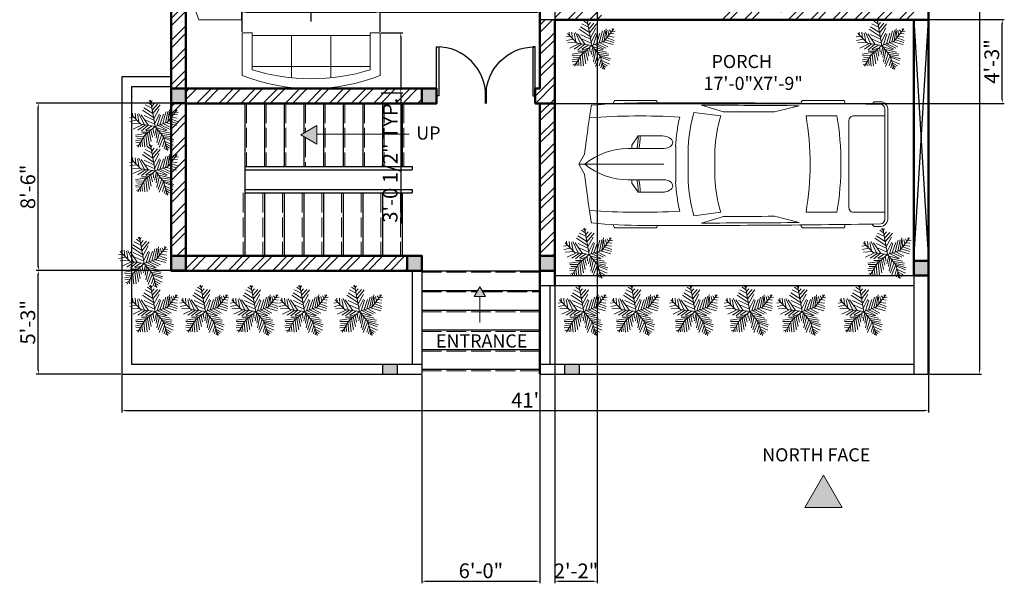
# Model space of a CAD drawing. Units: inches. Extents: x 381 to 1001, y 3003 to 3971.
# Tile 1 of 4: x 386 to 986, y 3003 to 3347. Entities that reach past the tile are written whole.
import ezdxf

# ---------------------------------------------------------------- set-up
doc = ezdxf.new("R2010")
doc.units = ezdxf.units.IN
doc.linetypes.add('ACAD_ISO02W100', pattern=[15, 12, -3])
for name, color, linetype, lineweight in [('A-ANNO-DIMS', 2, 'Continuous', 18), ('A-ANNO-SYMB', 7, 'Continuous', 18), ('A-ANNO-TEXT', 7, 'Continuous', 25), ('A-AREA-IDEN', 7, 'Continuous', 18), ('A-COLS', 7, 'Continuous', 50), ('A-DOOR', 4, 'Continuous', 25), ('A-FLOR', 7, 'Continuous', 25), ('A-FLOR-STRS', 7, 'Continuous', 25), ('A-FLOR-STRS-HIDN', 8, 'ACAD_ISO02W100', 13), ('A-FURN', 8, 'Continuous', 18), ('A-SITE-VEHI', 8, 'Continuous', 13), ('A-WALL', 7, 'Continuous', 50), ('A-WALL-PATT', 252, 'Continuous', 13), ('L-PLNT', 3, 'Continuous', 13), ('L-PLNT-BED', 8, 'Continuous', 25)]:
    doc.layers.add(name, color=color, linetype=linetype, lineweight=lineweight)
doc.styles.get("Standard").update_dxf_attribs({"font": 'arial.ttf'})
doc.dimstyles.new('ISO-25', dxfattribs={"dimtxt": 9, "dimasz": 2.5, "dimexe": 1.25, "dimexo": 0.625, "dimtad": 1, "dimlunit": 3, "dimtxsty": 'Standard', "dimcen": 2.5, "dimadec": 0, "dimazin": 0, "dimtfac": 1, "dimtmove": 0, "dimatfit": 3, "dimfxl": 1, "dimarcsym": 0})

# ---------------------------------------------------------------- blocks, each defined once
blk = doc.blocks.new('*U2')
for p, q in [((0, 0), (0, -6)), ((40, 0), (40, -6))]:
    blk.add_line(p, q)
blk.add_lwpolyline([(0, 0), (0, 40), (1.75, 40), (1.75, 0)], close=True)
blk.add_arc((0, 0), 40, 0, 90)
blk = doc.blocks.new('*U13')
for p, q in [((21.1, 37.41), (21.1, 36.83)), ((46.55, 38.89), (22.35, 38.89)), ((47.8, 37.39), (47.8, 37.41)), ((135.45, 37.07), (135.45, 37.41)), ((136.7, 38.89), (160.9, 38.89)), ((162.15, 37.41), (162.15, 36.77)), ((70.03, 31.54), (86.41, 29.35)), ((87.99, 31.87), (74.76, 35.92)), ((134.31, 35.6), (119.29, 31.78)), ((186.47, -33.5), (186.47, 33.5)), ((188.4, -32.76), (188.4, 32.76)), ((138.42, 29.35), (157.25, 29.35)), ((164.52, 26.39), (164.52, -26.39)), ((186.47, 29.35), (167.01, 29.35)), ((32.27, 11.63), (36.13, 17.17)), ((36.13, 17.17), (50.94, 17.17)), ((3.27, 6.13), (0.1, 0.41)), ((29.77, 9.51), (51.68, 9.51)), ((32.12, 9.51), (32.12, 11.15)), ((58.92, -10.77), (58.92, 10.77)), ((66.55, -10.53), (66.55, 10.53)), ((82.74, 8.5), (82.74, -8.5)), ((186.47, -10.53), (186.47, 10.53)), ((0, 0), (51.68, 0)), ((0.1, -0.41), (3.27, -6.13)), ((29.77, -9.51), (51.68, -9.51)), ((32.12, -9.51), (32.12, -11.15)), ((32.27, -11.63), (36.13, -17.17)), ((36.13, -17.17), (50.94, -17.17)), ((86.41, -29.35), (70.03, -31.54)), ((157.25, -29.35), (138.42, -29.35)), ((167.01, -29.35), (186.47, -29.35)), ((87.99, -31.87), (74.76, -35.92)), ((134.31, -35.6), (119.29, -31.78)), ((21.1, -37.41), (21.1, -36.83)), ((46.55, -38.89), (22.35, -38.89)), ((47.8, -37.39), (47.8, -37.41)), ((135.45, -37.07), (135.45, -37.41)), ((136.7, -38.89), (160.9, -38.89)), ((162.15, -37.41), (162.15, -36.77))]:
    blk.add_line(p, q)
for centre, major_axis, ratio, start_param, end_param in [((41.19, -490.86), (0, 528.23), 0.842304, 0.00281, 0.075598), ((22.35, 37.41), (0, -1.48), 0.842304, 3.141593, 4.712389), ((64.48, -10555.62), (0, 10593.03), 0.842304, -0.013397, 0.002797), ((46.55, 37.41), (0, 1.48), 0.842304, -1.570796, 0), ((136.7, 37.41), (0, -1.48), 0.842304, 3.141593, 4.712389), ((160.9, 37.41), (0, 1.48), 0.842304, -1.570796, 0), ((180.63, 35.84), (0, 2.22), 0.842304, -0.013017, 1.249894), ((64.48, -10556.36), (0, 10595.31), 0.842304, -0.013397, -0.013017), ((183.98, 33.5), (0, -2.96), 0.842304, 1.570796, 3.128196), ((183.98, 32.76), (0, -5.25), 0.842304, 1.570796, 3.128196), ((266.03, -27.52), (0, 313.31), 0.842304, 1.367076, 1.39176), ((135.29, 5.39), (0, 81.77), 0.842304, 1.245306, 1.50788), ((64.48, -10555.62), (0, -10591.55), 0.842304, 3.133765, 3.140441), ((95.79, -3666.35), (0, -3698.24), 0.842304, 3.134049, 3.144098), ((259.18, -27.52), (0, -305.3), 0.842304, 4.528606, 4.561838), ((37.47, -593.96), (0, -623.33), 0.842304, 3.096046, 3.200911), ((134.4, 5.39), (0, -89.78), 0.842304, 4.449482, 4.652344), ((149.6, 2.8), (0, -79.58), 0.842304, 4.372215, 4.640744), ((17.08, 0), (0, 147.02), 0.842304, 4.511394, 4.913384), ((35.91, 0), (0, 147.02), 0.842304, 4.511394, 4.913384), ((167.01, 26.39), (0, 2.96), 0.842304, 0, 1.570796), ((-204.49, 52.4), (0, -250.96), 0.842304, 1.385369, 1.434372), ((13.04, 17.01), (0, 27.42), 0.842304, 4.435146, 4.718221), ((14.2, 17.01), (0, 27.42), 0.842304, 4.435146, 4.718221), ((50.79, 13.34), (6.34, -0.36), 0.603834, -1.395552, 1.581315), ((29.77, -46.66), (0, 56.17), 0.842304, 0, 0.590319), ((32.75, 11.15), (0, 0.74), 0.842304, 0.879714, 1.570796), ((0.62, 0), (0, -0.74), 0.842304, 4.131459, 5.293319), ((29.77, 46.66), (0, 56.17), 0.842304, 2.551274, 3.141593), ((-204.49, -52.4), (0, 250.96), 0.842304, -1.434372, -1.385369), ((32.75, -11.15), (0, -0.74), 0.842304, 4.712389, 5.403472), ((13.04, -17.01), (0, -27.42), 0.842304, 1.564964, 1.848039), ((14.2, -17.01), (0, -27.42), 0.842304, 1.564964, 1.848039), ((134.4, -5.39), (0, -89.78), 0.842304, -1.510751, -1.307889), ((135.29, -5.39), (0, -81.77), 0.842304, -1.50788, -1.245306), ((149.6, -2.8), (0, -79.58), 0.842304, -1.499151, -1.230623), ((259.18, 27.52), (0, 305.3), 0.842304, 1.721348, 1.754579), ((266.03, 27.52), (0, 313.31), 0.842304, 1.749832, 1.774517), ((37.47, 593.96), (0, -623.33), 0.842304, -0.059319, 0.045547), ((167.01, -26.39), (0, -2.96), 0.842304, 4.712389, 6.283185), ((41.19, 490.86), (0, -528.23), 0.842304, -0.075598, -0.00281), ((64.48, 10555.62), (0, -10591.55), 0.842304, 0.001152, 0.007828), ((95.79, 3666.35), (0, -3698.24), 0.842304, -0.002505, 0.007544), ((183.98, -33.5), (0, 2.96), 0.842304, 3.15499, 4.712389), ((183.98, -32.76), (0, -5.25), 0.842304, 0.013397, 1.570796), ((22.35, -37.41), (0, 1.48), 0.842304, 1.570796, 3.141593), ((64.48, 10555.62), (0, 10593.03), 0.842304, 3.138796, 3.15499), ((46.55, -37.41), (0, -1.48), 0.842304, 0, 1.570796), ((136.7, -37.41), (0, -1.48), 0.842304, -1.570796, 0), ((160.9, -37.41), (0, 1.48), 0.842304, 3.141593, 4.712389), ((180.63, -35.84), (0, -2.22), 0.842304, -1.249894, 0.013017), ((64.48, 10556.36), (0, 10595.31), 0.842304, 3.15461, 3.15499)]:
    blk.add_ellipse(centre, major_axis=major_axis, ratio=ratio, start_param=start_param, end_param=end_param)
at = {"extrusion": (0, 0, -1)}
blk.add_ellipse((50.79, -13.34), major_axis=(6.34, 0.36), ratio=0.603834, start_param=-1.395552, end_param=1.581315, dxfattribs=at)
blk = doc.blocks.new('*U15')
for p, q in [((-7.288, 39.707), (-21.778, 46.673)), ((-8.737, 47.138), (-17.069, 52.711)), ((-10.186, 53.64), (-13.084, 55.962)), ((0, 0), (-10.5, 57)), ((-9.099, 51.782), (-6.563, 55.962)), ((-7.65, 43.423), (-2.578, 49.46)), ((-5.839, 35.992), (4.667, 48.067)), ((-5.114, 27.632), (10.463, 46.673)), ((-31.5, 4.5), (-52.5, 25.5)), ((-48.585, 21.131), (-49.309, 29.026)), ((-43.513, 28.561), (-42.427, 15.558)), ((-38.442, 26.239), (-34.819, 7.663)), ((-35.544, 28.097), (-24.314, 3.947)), ((-14.533, 2.09), (-30.834, 25.31)), ((-3.665, 19.273), (-27.574, 35.527)), ((-5.114, 28.097), (-24.676, 40.636)), ((-24.314, 23.917), (-2.941, 13.7)), ((-2.941, 16.486), (8.652, 37.85)), ((-1.129, 6.734), (9.014, 26.704)), ((3.942, 1.625), (11.187, 24.381)), ((10.101, 3.483), (17.708, 26.239)), ((16.259, 5.805), (23.142, 31.348)), ((22.055, 7.198), (27.489, 32.277)), ((27, 9), (48, 36)), ((27.127, 9.056), (31.112, 35.992)), ((31.836, 30.883), (32.561, 16.486)), ((35.096, 32.741), (37.27, 22.524)), ((38.719, 34.134), (41.979, 28.561)), ((40.53, 25.775), (48.862, 24.846)), ((43.791, 29.954), (51.036, 30.883)), ((44.153, 36.456), (45.239, 32.741)), ((-47.498, 19.737), (-55.83, 18.344)), ((-40.615, 13.7), (-55.105, 10.913)), ((-33.37, 6.269), (-52.207, 5.34)), ((-28.299, 3.483), (-47.86, -5.805)), ((-21.416, 3.018), (-38.079, -8.128)), ((0, 0), (-31.5, 4.5)), ((-15.982, 2.09), (-30.11, -9.521)), ((0, 0), (-22.5, -19.5)), ((-6.563, 1.161), (-21.416, -8.128)), ((-20.691, 13.7), (-1.129, 4.876)), ((0, 0), (27, 9)), ((0, 0), (18, -22.5)), ((6.478, 1.625), (26.04, -8.592)), ((11.187, 3.483), (30.749, -5.805)), ((18.07, 5.805), (35.096, -3.483)), ((24.229, 7.663), (46.688, 1.625)), ((29.662, 12.307), (48.137, 6.269)), ((33.285, 16.486), (48.862, 10.913)), ((36.183, 19.737), (48.137, 17.88)), ((-17.431, -15.094), (-42.789, -18.809)), ((-22.5, -19.5), (-37.5, -45)), ((-15.257, -12.772), (-30.11, -12.772)), ((-20.691, -18.345), (-17.793, -44.352)), ((-6.563, -5.805), (-19.967, -9.985)), ((-17.069, -15.094), (-12.721, -40.172)), ((-13.446, -11.378), (-8.737, -32.741)), ((-9.461, -8.592), (-6.201, -23.453)), ((-4.752, -3.483), (-3.665, -14.629)), ((2.493, -3.019), (-1.491, -20.202)), ((1.769, -2.555), (24.229, -9.521)), ((5.029, -6.27), (2.131, -25.775)), ((9.014, -11.378), (3.58, -35.992)), ((14.085, -16.951), (6.478, -40.172)), ((7.565, -9.056), (32.198, -14.629)), ((12.274, -15.094), (36.907, -18.809)), ((16.259, -19.738), (36.183, -22.989)), ((-28.299, -29.026), (-42.789, -31.348)), ((-24.314, -21.596), (-42.427, -22.06)), ((-30.834, -34.135), (-42.427, -35.528)), ((-34.457, -39.708), (-40.978, -42.494)), ((-26.849, -26.24), (-40.253, -25.775)), ((-32.646, -36.921), (-31.921, -44.352)), ((-29.023, -30.884), (-27.936, -43.887)), ((-25.038, -23.918), (-22.865, -45.281)), ((18.07, -22.524), (8.289, -45.745)), ((20.244, -30.419), (15.897, -44.816)), ((18, -22.5), (27, -52.5)), ((18.433, -22.524), (40.53, -29.026)), ((19.157, -25.311), (38.719, -33.206)), ((22.78, -37.85), (19.519, -48.532)), ((21.331, -32.741), (39.081, -40.636)), ((22.78, -38.314), (34.372, -44.816)), ((24.591, -45.745), (23.142, -50.854)), ((24.591, -43.423), (30.749, -47.603)), ((26.764, -49.925), (28.213, -50.854))]:
    blk.add_line(p, q)
blk = doc.blocks.new('Sofa - Roundback 7 ft.')
for p, q in [((-36.000027, -34), (-36.000027, -11.4696)), ((-12.00002, -32.4421), (-12.00003, -6.5971)), ((11.99997, -32.4421), (11.99998, -6.5971)), ((35.99998, -34), (35.99998, -11.4696)), ((-35.999844, -13.3819), (35.9998, -13.3819)), ((-36.000027, -32.4421), (35.99998, -32.4421))]:
    blk.add_line(p, q)
for points in [[(-36.000027, -34), (-42.000027, -34), (-42.000027, -8)], [(41.99998, -8), (41.99998, -34), (35.99998, -34)]]:
    blk.add_lwpolyline(points)
for centre, radius, start, end in [((0, -114.25), 114.25, 68.43141, 111.5686), ((-0.00001, -127.1968), 121.1968, 72.72033, 107.2797)]:
    blk.add_arc(centre, radius, start, end)
blk = doc.blocks.new('*D22')
at = {"layer": 'A-ANNO-DIMS', "color": 0, "lineweight": -2, "transparency": 16777216}
for p, q in [((940.7, 3889.64), (972.35, 3889.64)), ((971.1, 3887.14), (971.1, 3133.06)), ((940.7, 3130.56), (972.35, 3130.56))]:
    blk.add_line(p, q, dxfattribs=at)
at = {"layer": 'A-ANNO-DIMS', "color": 0, "transparency": 16777216}
for points in [[(970.69, 3887.14), (971.52, 3887.14), (971.1, 3889.64)], [(970.69, 3133.06), (971.52, 3133.06), (971.1, 3130.56)]]:
    blk.add_solid(points, dxfattribs=at)
at = {"layer": 'Defpoints', "color": 0, "transparency": 16777216}
for p in [(940.08, 3889.64), (940.08, 3130.56), (971.1, 3130.56)]:
    blk.add_point(p, dxfattribs=at)
at = {"layer": 'A-ANNO-DIMS', "color": 0, "transparency": 16777216, "insert": (965.88, 3510.1), "char_height": 9, "attachment_point": 5, "rotation": 90}
blk.add_mtext('63\'-3.07"', dxfattribs=at)
blk = doc.blocks.new('*D23')
at = {"layer": 'A-ANNO-DIMS', "color": 0, "lineweight": -2, "transparency": 16777216}
for p, q in [((448.08, 3129.94), (448.08, 3107.09)), ((940.08, 3129.94), (940.08, 3107.09)), ((450.58, 3108.34), (937.58, 3108.34))]:
    blk.add_line(p, q, dxfattribs=at)
at = {"layer": 'A-ANNO-DIMS', "color": 0, "transparency": 16777216}
for points in [[(450.58, 3108.76), (450.58, 3107.92), (448.08, 3108.34)], [(937.58, 3108.76), (937.58, 3107.92), (940.08, 3108.34)]]:
    blk.add_solid(points, dxfattribs=at)
at = {"layer": 'Defpoints', "color": 0, "transparency": 16777216}
for p in [(448.08, 3130.56), (940.08, 3130.56), (940.08, 3108.34)]:
    blk.add_point(p, dxfattribs=at)
at = {"layer": 'A-ANNO-DIMS', "color": 0, "transparency": 16777216, "insert": (694.08, 3113.48), "char_height": 9, "attachment_point": 5}
blk.add_mtext("41'", dxfattribs=at)
blk = doc.blocks.new('COLUMN-9X9')
h = blk.add_hatch(color=256)
h.dxf.hatch_style = 1
h.paths.add_polyline_path([(9, 9), (0, 9), (0, 0), (9, 0)])
blk.add_lwpolyline([(0, 9), (9, 9), (9, 0), (0, 0)], close=True)
blk = doc.blocks.new('*D38')
at = {"layer": 'A-ANNO-DIMS', "color": 0, "lineweight": -2, "transparency": 16777216}
for p, q in [((521.58, 3339.19), (521.58, 3352.41)), ((524.08, 3351.16), (603.08, 3351.16)), ((605.58, 3339.19), (605.58, 3352.41)), ((605.58, 3351.16), (701.87, 3351.16))]:
    blk.add_line(p, q, dxfattribs=at)
at = {"layer": 'A-ANNO-DIMS', "color": 0, "transparency": 16777216}
for points in [[(524.08, 3351.58), (524.08, 3350.75), (521.58, 3351.16)], [(603.08, 3351.58), (603.08, 3350.75), (605.58, 3351.16)]]:
    blk.add_solid(points, dxfattribs=at)
at = {"layer": 'Defpoints', "color": 0, "transparency": 16777216}
for p in [(605.58, 3351.16), (521.58, 3338.56), (605.58, 3338.56)]:
    blk.add_point(p, dxfattribs=at)
at = {"layer": 'A-ANNO-DIMS', "color": 0, "transparency": 16777216, "insert": (654.97, 3356.45), "char_height": 9, "attachment_point": 5}
blk.add_mtext('SOFA 7\'-0" TYP.', dxfattribs=at)
blk = doc.blocks.new('*D39')
at = {"layer": 'A-ANNO-DIMS', "color": 0, "lineweight": -2, "transparency": 16777216}
for p, q in [((606.2, 3338.56), (619.43, 3338.56)), ((618.18, 3336.06), (618.18, 3304.4)), ((606.2, 3301.9), (619.43, 3301.9)), ((618.18, 3301.9), (618.18, 3222.32))]:
    blk.add_line(p, q, dxfattribs=at)
at = {"layer": 'A-ANNO-DIMS', "color": 0, "transparency": 16777216}
for points in [[(617.76, 3336.06), (618.59, 3336.06), (618.18, 3338.56)], [(617.76, 3304.4), (618.59, 3304.4), (618.18, 3301.9)]]:
    blk.add_solid(points, dxfattribs=at)
at = {"layer": 'Defpoints', "color": 0, "transparency": 16777216}
for p in [(605.58, 3338.56), (605.58, 3301.9), (618.18, 3301.9)]:
    blk.add_point(p, dxfattribs=at)
at = {"layer": 'A-ANNO-DIMS', "color": 0, "transparency": 16777216, "insert": (612.9, 3260.86), "char_height": 9, "attachment_point": 5, "rotation": 90}
blk.add_mtext('3\'-0 1/2" TYP.', dxfattribs=at)
blk = doc.blocks.new('*D55')
at = {"layer": 'A-ANNO-DIMS', "color": 0, "lineweight": -2, "transparency": 16777216}
for p, q in [((631.08, 3129.94), (631.08, 3002.98)), ((703.08, 3129.94), (703.08, 3002.98)), ((633.58, 3004.23), (700.58, 3004.23))]:
    blk.add_line(p, q, dxfattribs=at)
at = {"layer": 'A-ANNO-DIMS', "color": 0, "transparency": 16777216}
for points in [[(633.58, 3004.64), (633.58, 3003.81), (631.08, 3004.23)], [(700.58, 3004.64), (700.58, 3003.81), (703.08, 3004.23)]]:
    blk.add_solid(points, dxfattribs=at)
at = {"layer": 'Defpoints', "color": 0, "transparency": 16777216}
for p in [(631.08, 3130.56), (703.08, 3130.56), (703.08, 3004.23)]:
    blk.add_point(p, dxfattribs=at)
at = {"layer": 'A-ANNO-DIMS', "color": 0, "transparency": 16777216, "insert": (667.08, 3009.45), "char_height": 9, "attachment_point": 5}
blk.add_mtext('6\'-0"', dxfattribs=at)
blk = doc.blocks.new('*D56')
at = {"layer": 'A-ANNO-DIMS', "color": 0, "lineweight": -2, "transparency": 16777216}
for p, q in [((477.45, 3295.64), (395.91, 3295.64)), ((397.16, 3196.14), (397.16, 3293.14)), ((477.45, 3193.64), (395.91, 3193.64))]:
    blk.add_line(p, q, dxfattribs=at)
at = {"layer": 'A-ANNO-DIMS', "color": 0, "transparency": 16777216}
for points in [[(396.74, 3293.14), (397.57, 3293.14), (397.16, 3295.64)], [(396.74, 3196.14), (397.57, 3196.14), (397.16, 3193.64)]]:
    blk.add_solid(points, dxfattribs=at)
at = {"layer": 'Defpoints', "color": 0, "transparency": 16777216}
for p in [(397.16, 3295.64), (478.08, 3295.64), (478.08, 3193.64)]:
    blk.add_point(p, dxfattribs=at)
at = {"layer": 'A-ANNO-DIMS', "color": 0, "transparency": 16777216, "insert": (391.94, 3244.64), "char_height": 9, "attachment_point": 5, "rotation": 90}
blk.add_mtext('8\'-6"', dxfattribs=at)
blk = doc.blocks.new('*D57')
at = {"layer": 'A-ANNO-DIMS', "color": 0, "lineweight": -2, "transparency": 16777216}
for p, q in [((703.7, 3346.64), (986.28, 3346.64)), ((985.03, 3298.06), (985.03, 3344.14)), ((703.7, 3295.56), (986.28, 3295.56))]:
    blk.add_line(p, q, dxfattribs=at)
at = {"layer": 'A-ANNO-DIMS', "color": 0, "transparency": 16777216}
for points in [[(984.61, 3344.14), (985.44, 3344.14), (985.03, 3346.64)], [(984.61, 3298.06), (985.44, 3298.06), (985.03, 3295.56)]]:
    blk.add_solid(points, dxfattribs=at)
at = {"layer": 'Defpoints', "color": 0, "transparency": 16777216}
for p in [(703.08, 3346.64), (985.03, 3346.64), (703.08, 3295.56)]:
    blk.add_point(p, dxfattribs=at)
at = {"layer": 'A-ANNO-DIMS', "color": 0, "transparency": 16777216, "insert": (979.81, 3321.1), "char_height": 9, "attachment_point": 5, "rotation": 90}
blk.add_mtext('4\'-3"', dxfattribs=at)
blk = doc.blocks.new('*D58')
at = {"layer": 'A-ANNO-DIMS', "color": 0, "lineweight": -2, "transparency": 16777216}
for p, q in [((477.45, 3193.64), (395.91, 3193.64)), ((397.16, 3133.06), (397.16, 3191.14)), ((447.45, 3130.56), (395.91, 3130.56))]:
    blk.add_line(p, q, dxfattribs=at)
at = {"layer": 'A-ANNO-DIMS', "color": 0, "transparency": 16777216}
for points in [[(396.74, 3191.14), (397.57, 3191.14), (397.16, 3193.64)], [(396.74, 3133.06), (397.57, 3133.06), (397.16, 3130.56)]]:
    blk.add_solid(points, dxfattribs=at)
at = {"layer": 'Defpoints', "color": 0, "transparency": 16777216}
for p in [(397.16, 3193.64), (478.08, 3193.64), (448.08, 3130.56)]:
    blk.add_point(p, dxfattribs=at)
at = {"layer": 'A-ANNO-DIMS', "color": 0, "transparency": 16777216, "insert": (391.93, 3162.1), "char_height": 9, "attachment_point": 5, "rotation": 90}
blk.add_mtext('5\'-3"', dxfattribs=at)
blk = doc.blocks.new('*D59')
at = {"layer": 'A-ANNO-DIMS', "color": 0, "lineweight": -2, "transparency": 16777216}
for p, q in [((712.08, 3502.01), (712.08, 3002.98)), ((738.08, 3501.94), (738.08, 3002.98)), ((714.58, 3004.23), (735.58, 3004.23))]:
    blk.add_line(p, q, dxfattribs=at)
at = {"layer": 'A-ANNO-DIMS', "color": 0, "transparency": 16777216}
for points in [[(714.58, 3004.64), (714.58, 3003.81), (712.08, 3004.23)], [(735.58, 3004.64), (735.58, 3003.81), (738.08, 3004.23)]]:
    blk.add_solid(points, dxfattribs=at)
at = {"layer": 'Defpoints', "color": 0, "transparency": 16777216}
for p in [(712.08, 3502.64), (738.08, 3502.56), (738.08, 3004.23)]:
    blk.add_point(p, dxfattribs=at)
at = {"layer": 'A-ANNO-DIMS', "color": 0, "transparency": 16777216, "insert": (725.08, 3009.37), "char_height": 9, "attachment_point": 5}
blk.add_mtext('2\'-2"', dxfattribs=at)
blk = doc.blocks.new('*D61')
at = {"layer": 'A-ANNO-DIMS', "color": 0, "lineweight": -2, "transparency": 16777216}
for p, q in [((563.58, 3569.42), (563.58, 3469.06)), ((563.58, 3345.37), (563.58, 3466.56))]:
    blk.add_line(p, q, dxfattribs=at)
at = {"layer": 'A-ANNO-DIMS', "color": 0, "transparency": 16777216}
blk.add_solid([(563.99, 3469.06), (563.16, 3469.06), (563.58, 3466.56)], dxfattribs=at)
at = {"layer": 'Defpoints', "color": 0, "transparency": 16777216}
for p in [(563.58, 3466.56), (563.58, 3345.37)]:
    blk.add_point(p, dxfattribs=at)
at = {"layer": 'A-ANNO-DIMS', "color": 0, "transparency": 16777216, "insert": (568.8, 3539.28), "char_height": 9, "attachment_point": 5, "rotation": 270.00014}
blk.add_mtext('2X R10\'-1"', dxfattribs=at)

msp = doc.modelspace()

# ---------------------------------------------------------------- hatches: boundary and pattern name
at = {"layer": 'A-ANNO-SYMB'}
h = msp.add_hatch(color=256, dxfattribs=at)
h.dxf.hatch_style = 1
h.paths.add_polyline_path([(666.485, 3183.741), (663.054, 3177.797), (669.917, 3177.797)])
h.paths.add_polyline_path([(567.007, 3282.075), (557.207, 3276.417), (567.007, 3270.759)])
h = msp.add_hatch(color=256, dxfattribs=at)
h.dxf.hatch_style = 1
h.paths.add_polyline_path([(876.009, 3068.86), (864.644, 3049.176), (887.373, 3049.176)])
h.paths.add_polyline_path([(727.078, 3136.565), (718.078, 3136.565), (718.078, 3130.565), (727.078, 3130.565)])
h.paths.add_polyline_path([(616.078, 3136.565), (607.078, 3136.565), (607.078, 3130.565), (616.078, 3130.565)])
at = {"layer": 'A-WALL-PATT'}
h = msp.add_hatch(dxfattribs=at)
h.set_pattern_fill('ANSI32', color=256)
h.paths.add_polyline_path([(652.078, 3667.565), (487.078, 3667.565), (487.078, 3658.565), (631.078, 3658.565), (631.078, 3655.565), (634.678, 3655.565), (640.078, 3655.565), (640.078, 3658.565), (652.078, 3658.565)])
h.paths.add_polyline_path([(487.078, 3658.637), (478.078, 3658.637), (478.078, 3634.565), (487.078, 3634.565)])
h.paths.add_polyline_path([(487.078, 3703.565), (478.078, 3703.565), (478.078, 3667.637), (487.078, 3667.637)])
h.paths.add_polyline_path([(661.078, 3811.637), (652.078, 3811.637), (652.078, 3706.565), (661.078, 3706.565)])
h.paths.add_polyline_path([(661.078, 3670.565), (655.678, 3670.565), (652.078, 3670.565), (652.078, 3667.637), (661.078, 3667.637)])
h.paths.add_polyline_path([(487.078, 3811.637), (478.078, 3811.637), (478.078, 3775.565), (487.078, 3775.565)])
h.paths.add_polyline_path([(487.078, 3880.565), (478.078, 3880.565), (478.078, 3820.637), (487.078, 3820.637)])
h.paths.add_polyline_path([(661.078, 3880.637), (652.078, 3880.637), (652.078, 3820.637), (661.078, 3820.637)])
h.paths.add_polyline_path([(652.078, 3820.565), (568.078, 3820.565), (568.078, 3823.565), (563.578, 3823.565), (562.078, 3823.565), (562.078, 3820.565), (559.078, 3820.565), (559.078, 3811.565), (652.078, 3811.565), (652.078, 3811.637)])
h.paths.add_polyline_path([(523.078, 3820.565), (487.078, 3820.565), (487.078, 3811.565), (523.078, 3811.565)])
h.paths.add_polyline_path([(619.798, 3889.565), (487.078, 3889.565), (487.078, 3880.565), (562.078, 3880.565), (562.078, 3853.565), (568.078, 3853.565), (568.078, 3880.565), (619.798, 3880.565)])
h.paths.add_polyline_path([(652.078, 3889.565), (640.798, 3889.565), (640.798, 3880.565), (652.078, 3880.565), (652.078, 3880.637)])
h.paths.add_polyline_path([(757.078, 3889.565), (661.078, 3889.565), (661.078, 3880.565), (757.078, 3880.565)])
h.paths.add_polyline_path([(766.078, 3880.637), (757.078, 3880.637), (757.078, 3820.637), (766.078, 3820.637)])
h.paths.add_polyline_path([(773.578, 3889.565), (766.078, 3889.565), (766.078, 3880.565), (773.578, 3880.565)])
h.paths.add_polyline_path([(931.078, 3889.565), (794.578, 3889.565), (794.578, 3880.565), (850.078, 3880.565), (850.078, 3853.565), (856.078, 3853.565), (856.078, 3880.565), (931.078, 3880.565)])
h.paths.add_polyline_path([(859.078, 3820.565), (856.078, 3820.565), (856.078, 3823.565), (850.078, 3823.565), (850.078, 3820.565), (766.078, 3820.565), (766.078, 3811.565), (859.078, 3811.565)])
h.paths.add_polyline_path([(940.078, 3880.637), (931.078, 3880.637), (931.078, 3820.637), (940.078, 3820.637)])
h.paths.add_polyline_path([(931.078, 3820.565), (895.078, 3820.565), (895.078, 3811.565), (931.078, 3811.565)])
h.paths.add_polyline_path([(940.078, 3811.637), (931.078, 3811.637), (931.078, 3775.565), (940.078, 3775.565)])
h.paths.add_polyline_path([(766.078, 3811.637), (757.078, 3811.637), (757.078, 3706.565), (766.078, 3706.565)])
h.paths.add_polyline_path([(940.078, 3703.565), (931.078, 3703.565), (931.078, 3667.637), (940.078, 3667.637)])
h.paths.add_polyline_path([(931.078, 3667.565), (766.078, 3667.565), (766.078, 3658.565), (931.078, 3658.565)])
h.paths.add_polyline_path([(940.078, 3658.637), (931.078, 3658.637), (931.078, 3621.065), (940.078, 3621.065)])
h.paths.add_polyline_path([(940.078, 3549.065), (931.078, 3549.065), (931.078, 3511.637), (940.078, 3511.637)])
h.paths.add_polyline_path([(931.078, 3511.565), (847.078, 3511.565), (847.078, 3502.565), (931.078, 3502.565)])
h.paths.add_polyline_path([(802.078, 3511.565), (712.078, 3511.565), (712.078, 3502.565), (802.078, 3502.565)])
h.paths.add_polyline_path([(712.078, 3502.637), (703.078, 3502.637), (703.078, 3355.637), (712.078, 3355.637)])
h.paths.add_polyline_path([(740.578, 3355.565), (712.078, 3355.565), (712.078, 3346.565), (740.578, 3346.565)])
h.paths.add_polyline_path([(841.078, 3355.565), (812.578, 3355.565), (812.578, 3346.565), (841.078, 3346.565)])
h.paths.add_polyline_path([(850.078, 3412.565), (841.078, 3412.565), (841.078, 3355.637), (850.078, 3355.637)], flags=17)
h.paths.add_polyline_path([(940.078, 3502.637), (931.078, 3502.637), (931.078, 3454.565), (841.078, 3454.565), (841.078, 3442.565), (850.078, 3442.565), (850.078, 3445.565), (931.078, 3445.565), (931.078, 3355.637), (940.078, 3355.637)])
h.paths.add_polyline_path([(931.078, 3355.565), (850.078, 3355.565), (850.078, 3346.565), (931.078, 3346.565)])
h.paths.add_polyline_path([(712.078, 3346.637), (703.078, 3346.637), (703.078, 3304.565), (700.078, 3304.565), (700.078, 3295.565), (712.078, 3295.565)])
h.paths.add_polyline_path([(622.078, 3202.565), (487.078, 3202.565), (487.078, 3193.565), (622.078, 3193.565)])
h.paths.add_polyline_path([(487.078, 3295.637), (478.078, 3295.637), (478.078, 3202.637), (487.078, 3202.637)])
h.paths.add_polyline_path([(712.078, 3295.565), (703.078, 3295.565), (703.078, 3202.565), (712.078, 3202.565)])
h = msp.add_hatch(dxfattribs=at)
h.set_pattern_fill('ANSI32', color=256)
h.paths.add_polyline_path([(487.078, 3352.565), (478.078, 3352.565), (478.078, 3304.637), (487.078, 3304.637)])
h.paths.add_polyline_path([(631.078, 3304.565), (487.078, 3304.565), (487.078, 3295.565), (631.078, 3295.565)])
h.paths.add_polyline_path([(487.078, 3472.637), (478.078, 3472.637), (478.078, 3424.565), (487.078, 3424.565)])
h.paths.add_polyline_path([(631.078, 3481.565), (592.078, 3481.565), (592.078, 3496.565), (583.078, 3496.565), (583.078, 3481.565), (487.078, 3481.565), (487.078, 3472.565), (631.078, 3472.565)])
h.paths.add_polyline_path([(487.078, 3562.565), (478.078, 3562.565), (478.078, 3538.637), (487.078, 3538.637)])
h.paths.add_polyline_path([(487.078, 3529.637), (478.078, 3529.637), (478.078, 3516.065), (487.078, 3516.065)])
h.paths.add_polyline_path([(487.078, 3495.065), (478.078, 3495.065), (478.078, 3481.637), (487.078, 3481.637)])
h.paths.add_polyline_path([(631.078, 3538.565), (487.078, 3538.565), (487.078, 3529.565), (583.078, 3529.565), (583.078, 3526.565), (587.578, 3526.565), (592.078, 3526.565), (592.078, 3529.565), (631.078, 3529.565)])
h.paths.add_polyline_path([(640.078, 3619.565), (631.078, 3619.565), (631.078, 3538.565), (640.078, 3538.565)])

# ---------------------------------------------------------------- linework, layer by layer
at = {"layer": 'A-ANNO-SYMB'}
for p, q in [((623.391, 3276.703), (567.007, 3276.703)), ((666.476, 3162.015), (666.476, 3177.797))]:
    msp.add_line(p, q, dxfattribs=at)
for points in [[(557.207, 3276.417), (567.007, 3270.759), (567.007, 3282.075)], [(666.485, 3183.741), (663.054, 3177.797), (669.917, 3177.797)], [(876.009, 3068.86), (864.644, 3049.176), (887.373, 3049.176)]]:
    msp.add_lwpolyline(points, close=True, dxfattribs=at)
at = {"layer": 'A-FLOR'}
for p, q in [((931.078, 3346.565), (940.078, 3199.565)), ((931.078, 3199.565), (940.078, 3346.565)), ((931.078, 3199.565), (940.078, 3199.565)), ((712.078, 3190.565), (940.078, 3190.565)), ((703.078, 3184.565), (931.078, 3184.565))]:
    msp.add_line(p, q, dxfattribs=at)
at = {"layer": 'A-FLOR-STRS'}
for p, q in [((523.078, 3295.565), (523.078, 3243.065)), ((535.078, 3295.565), (535.078, 3257.065)), ((547.078, 3295.565), (547.078, 3257.065)), ((559.078, 3295.565), (559.078, 3277.497)), ((571.078, 3295.565), (571.078, 3257.065)), ((583.078, 3295.565), (583.078, 3257.065)), ((595.078, 3295.565), (595.078, 3257.065)), ((607.078, 3295.565), (607.078, 3257.065)), ((619.078, 3295.565), (619.078, 3257.065)), ((559.078, 3275.337), (559.078, 3257.065)), ((523.078, 3257.065), (625.078, 3257.065)), ((523.078, 3255.065), (625.078, 3255.065)), ((625.078, 3257.065), (625.078, 3255.065)), ((523.078, 3243.065), (625.078, 3243.065)), ((523.078, 3243.065), (523.078, 3202.565)), ((625.078, 3243.065), (625.078, 3241.065)), ((523.078, 3241.065), (625.078, 3241.065)), ((535.078, 3241.065), (535.078, 3202.565)), ((547.078, 3241.065), (547.078, 3202.565)), ((559.078, 3241.065), (559.078, 3202.565)), ((571.078, 3241.065), (571.078, 3202.565)), ((583.078, 3241.065), (583.078, 3202.565)), ((595.078, 3241.065), (595.078, 3202.565)), ((607.078, 3241.065), (607.078, 3202.565)), ((619.078, 3241.065), (619.078, 3202.565)), ((631.078, 3202.565), (631.078, 3130.565)), ((631.078, 3193.565), (703.078, 3193.565)), ((631.078, 3181.565), (665.229, 3181.565)), ((667.741, 3181.565), (703.078, 3181.565)), ((631.078, 3169.565), (703.078, 3169.565)), ((631.078, 3157.565), (703.078, 3157.565)), ((631.078, 3145.565), (703.078, 3145.565)), ((631.078, 3133.565), (703.078, 3133.565))]:
    msp.add_line(p, q, dxfattribs=at)
at = {"layer": 'A-FLOR-STRS-HIDN'}
for p, q in [((524.078, 3295.565), (524.078, 3257.065)), ((536.078, 3295.565), (536.078, 3257.065)), ((548.078, 3295.565), (548.078, 3257.065)), ((560.078, 3295.565), (560.078, 3278.074)), ((572.078, 3295.565), (572.078, 3257.065)), ((584.078, 3295.565), (584.078, 3257.065)), ((596.078, 3295.565), (596.078, 3257.065)), ((608.078, 3295.565), (608.078, 3257.065)), ((620.078, 3295.565), (620.078, 3257.065)), ((560.078, 3274.759), (560.078, 3257.065)), ((522.078, 3241.065), (522.078, 3202.565)), ((534.078, 3241.065), (534.078, 3202.565)), ((546.078, 3241.065), (546.078, 3202.565)), ((558.078, 3241.065), (558.078, 3202.565)), ((570.078, 3241.065), (570.078, 3202.565)), ((582.078, 3241.065), (582.078, 3202.565)), ((594.078, 3241.065), (594.078, 3202.565)), ((606.078, 3241.065), (606.078, 3202.565)), ((618.078, 3241.065), (618.078, 3202.565)), ((631.078, 3192.565), (703.078, 3192.565)), ((631.078, 3180.565), (664.652, 3180.565)), ((668.319, 3180.565), (703.078, 3180.565)), ((631.078, 3168.565), (703.078, 3168.565)), ((631.078, 3156.565), (703.078, 3156.565)), ((631.078, 3144.565), (703.078, 3144.565)), ((631.078, 3132.565), (703.078, 3132.565))]:
    msp.add_line(p, q, dxfattribs=at)
at = {"layer": 'A-WALL'}
for p, q in [((478.078, 3889.565), (478.078, 3193.565)), ((940.078, 3889.565), (940.078, 3130.565)), ((703.078, 3511.565), (703.078, 3304.565)), ((487.078, 3472.565), (487.078, 3304.565)), ((712.078, 3346.565), (940.078, 3346.565)), ((712.078, 3346.565), (712.078, 3184.565)), ((931.078, 3346.565), (931.078, 3193.565)), ((487.078, 3304.565), (640.078, 3304.565)), ((640.078, 3304.565), (640.078, 3295.565)), ((670.078, 3304.565), (670.078, 3295.565)), ((700.078, 3304.565), (700.078, 3295.565)), ((700.078, 3304.565), (703.078, 3304.565)), ((487.078, 3295.565), (640.078, 3295.565)), ((487.078, 3295.565), (487.078, 3202.565)), ((700.078, 3295.565), (712.078, 3295.565)), ((703.078, 3295.565), (703.078, 3130.565)), ((487.078, 3202.565), (631.078, 3202.565)), ((478.078, 3193.565), (631.078, 3193.565))]:
    msp.add_line(p, q, dxfattribs=at)
at = {"layer": 'L-PLNT-BED'}
for p, q in [((478.078, 3311.693), (448.078, 3311.693)), ((448.078, 3311.693), (448.078, 3130.565)), ((478.078, 3305.693), (454.078, 3305.693)), ((454.078, 3305.693), (454.078, 3136.565)), ((625.078, 3193.565), (625.078, 3136.565)), ((931.078, 3193.565), (931.078, 3130.565)), ((709.078, 3184.565), (709.078, 3136.565)), ((454.078, 3136.565), (631.078, 3136.565)), ((607.078, 3136.565), (607.078, 3130.565)), ((616.078, 3136.565), (616.078, 3130.565)), ((703.078, 3136.565), (931.078, 3136.565)), ((718.078, 3136.565), (718.078, 3130.565)), ((727.078, 3136.565), (727.078, 3130.565)), ((448.078, 3130.565), (631.078, 3130.565)), ((703.078, 3130.565), (940.078, 3130.565))]:
    msp.add_line(p, q, dxfattribs=at)

# ---------------------------------------------------------------- block references
at = {"layer": 'A-COLS'}
for p in [(478.078, 3295.637), (631.078, 3295.565), (478.078, 3193.637), (622.078, 3193.565), (703.078, 3193.565), (931.078, 3190.565)]:
    msp.add_blockref('COLUMN-9X9', p, dxfattribs=at)
at = {"layer": 'A-DOOR', "xscale": 0.75, "yscale": 0.75, "zscale": 0.75}
msp.add_blockref('*U2', (640.078, 3300.065), dxfattribs=at)
at = {"layer": 'A-DOOR', "xscale": -0.75, "yscale": 0.75, "zscale": 0.75, "rotation": 359.9999999999986}
msp.add_blockref('*U2', (700.078, 3300.065), dxfattribs=at)
at = {"layer": 'A-FURN', "rotation": 89.99998708239097}
msp.add_blockref('Sofa - Roundback 7 ft.', (487.078, 3388.565), dxfattribs=at)
at = {"layer": 'A-FURN', "xscale": -1, "rotation": 180}
msp.add_blockref('Sofa - Roundback 7 ft.', (563.578, 3304.565), dxfattribs=at)
at = {"layer": 'A-SITE-VEHI'}
msp.add_blockref('*U13', (726.936, 3258.517), dxfattribs=at)
at = {"layer": 'L-PLNT', "xscale": 0.2802404577001134, "yscale": 0.2802404577001134, "zscale": 0.2802404577001134}
for p in [(734.683, 3330.914), (911.589, 3330.914), (468.446, 3281.537), (468.446, 3254.33), (733.159, 3203.413), (915.08, 3203.413), (461.764, 3198.007), (468.446, 3168.703), (499.108, 3168.703), (529.799, 3168.703), (559.574, 3168.703), (592.985, 3168.703), (729.821, 3168.703), (761.743, 3168.703), (797.656, 3168.703), (831.175, 3168.703), (863.098, 3168.703), (900.607, 3168.703)]:
    msp.add_blockref('*U15', p, dxfattribs=at)

# ---------------------------------------------------------------- texts
at = {"layer": 'A-ANNO-TEXT', "char_height": 8, "attachment_point": 1}
for s, width, insert in [('UP', 14.79911, (627.659, 3281.47)), ('ENTRANCE', 64.05626, (639.659, 3154.721)), ('NORTH FACE', 74.63083, (838.631, 3085.296))]:
    msp.add_mtext_dynamic_manual_height_columns(s, width=width, gutter_width=12.5, heights=[0], dxfattribs=dict(at, insert=insert))
at = {"layer": 'A-AREA-IDEN', "insert": (802.854, 3325.08), "char_height": 8, "attachment_point": 1}
msp.add_mtext_dynamic_manual_height_columns('  PORCH\\P17\'-0"X7\'-9"', width=56.51599, gutter_width=12.5, heights=[0], dxfattribs=at)

# ---------------------------------------------------------------- dimensions: what is measured, and where the dimension line sits
at = {"layer": 'A-ANNO-DIMS'}
for base, p1, p2, override, picture, middle in [((971.102, 3130.565), (940.078, 3889.637), (940.078, 3130.565), {"dimclrd": 0, "dimclre": 0, "dimclrt": 0}, '*D22', (965.879, 3510.101)), ((985.028, 3346.637), (703.078, 3295.565), (703.078, 3346.637), {"dimdec": 1, "dimlfac": 1, "dimrnd": 0, "dimzin": 1, "dimdsep": 46, "dimlunit": 4, "dimfrac": 2}, '*D57', (979.805, 3321.101)), ((397.157, 3295.637), (478.078, 3193.637), (478.078, 3295.637), {"dimdec": 1, "dimlfac": 1, "dimrnd": 0, "dimzin": 1, "dimdsep": 46, "dimlunit": 4, "dimfrac": 2}, '*D56', (391.936, 3244.637)), ((397.157, 3193.637), (448.078, 3130.565), (478.078, 3193.637), {"dimdec": 1, "dimlfac": 1, "dimrnd": 0, "dimzin": 1, "dimdsep": 46, "dimlunit": 4, "dimfrac": 2}, '*D58', (391.933, 3162.101))]:
    dim = msp.add_linear_dim(base=base, p1=p1, p2=p2, angle=90, dimstyle='ISO-25', override=override, dxfattribs=at)
    dim.commit()
    dim.dimension.update_dxf_attribs({"geometry": picture, "text_midpoint": middle})
dim = msp.add_radius_dim(center=(563.578, 3345.368), mpoint=(563.578, 3466.565), text='2X <>', dimstyle='ISO-25', override={"dimdec": 1, "dimlfac": 1, "dimrnd": 0, "dimzin": 1, "dimdsep": 46, "dimlunit": 4, "dimfrac": 2}, dxfattribs=at)
dim.commit()
dim.dimension.update_dxf_attribs({"geometry": '*D61', "text_midpoint": (563.578, 3539.283), "dimtype": 164})
for base, p1, p2, override, picture, middle in [((738.078, 3004.226), (712.078, 3502.637), (738.078, 3502.565), {"dimdec": 1, "dimlfac": 1, "dimrnd": 0, "dimzin": 1, "dimdsep": 46, "dimlunit": 4, "dimfrac": 2}, '*D59', (725.078, 3009.37)), ((940.078, 3108.339), (448.078, 3130.565), (940.078, 3130.565), {"dimclrd": 0, "dimclre": 0, "dimclrt": 0}, '*D23', (694.078, 3113.482)), ((703.078, 3004.226), (631.078, 3130.565), (703.078, 3130.565), {"dimdec": 1, "dimlfac": 1, "dimrnd": 0, "dimzin": 1, "dimdsep": 46, "dimlunit": 4, "dimfrac": 2}, '*D55', (667.078, 3009.446))]:
    dim = msp.add_linear_dim(base=base, p1=p1, p2=p2, dimstyle='ISO-25', override=override, dxfattribs=at)
    dim.commit()
    dim.dimension.update_dxf_attribs({"geometry": picture, "text_midpoint": middle})
dim = msp.add_linear_dim(base=(605.578, 3351.165), p1=(521.578, 3338.565), p2=(605.578, 3338.565), text='SOFA <> TYP.', dimstyle='ISO-25', override={"dimdec": 1, "dimlfac": 1, "dimrnd": 0, "dimzin": 1, "dimdsep": 46, "dimlunit": 4, "dimfrac": 2}, dxfattribs=at)
dim.commit()
dim.dimension.update_dxf_attribs({"geometry": '*D38', "text_midpoint": (654.974, 3356.446)})
dim = msp.add_linear_dim(base=(618.178, 3301.898), p1=(605.578, 3338.565), p2=(605.578, 3301.898), angle=270, text='<> TYP.', dimstyle='ISO-25', override={"dimdec": 1, "dimlfac": 1, "dimrnd": 0, "dimzin": 1, "dimdsep": 46, "dimlunit": 4, "dimfrac": 2}, dxfattribs=at)
dim.commit()
dim.dimension.update_dxf_attribs({"geometry": '*D39', "text_midpoint": (612.897, 3260.861)})

doc.saveas('drawing.dxf')
